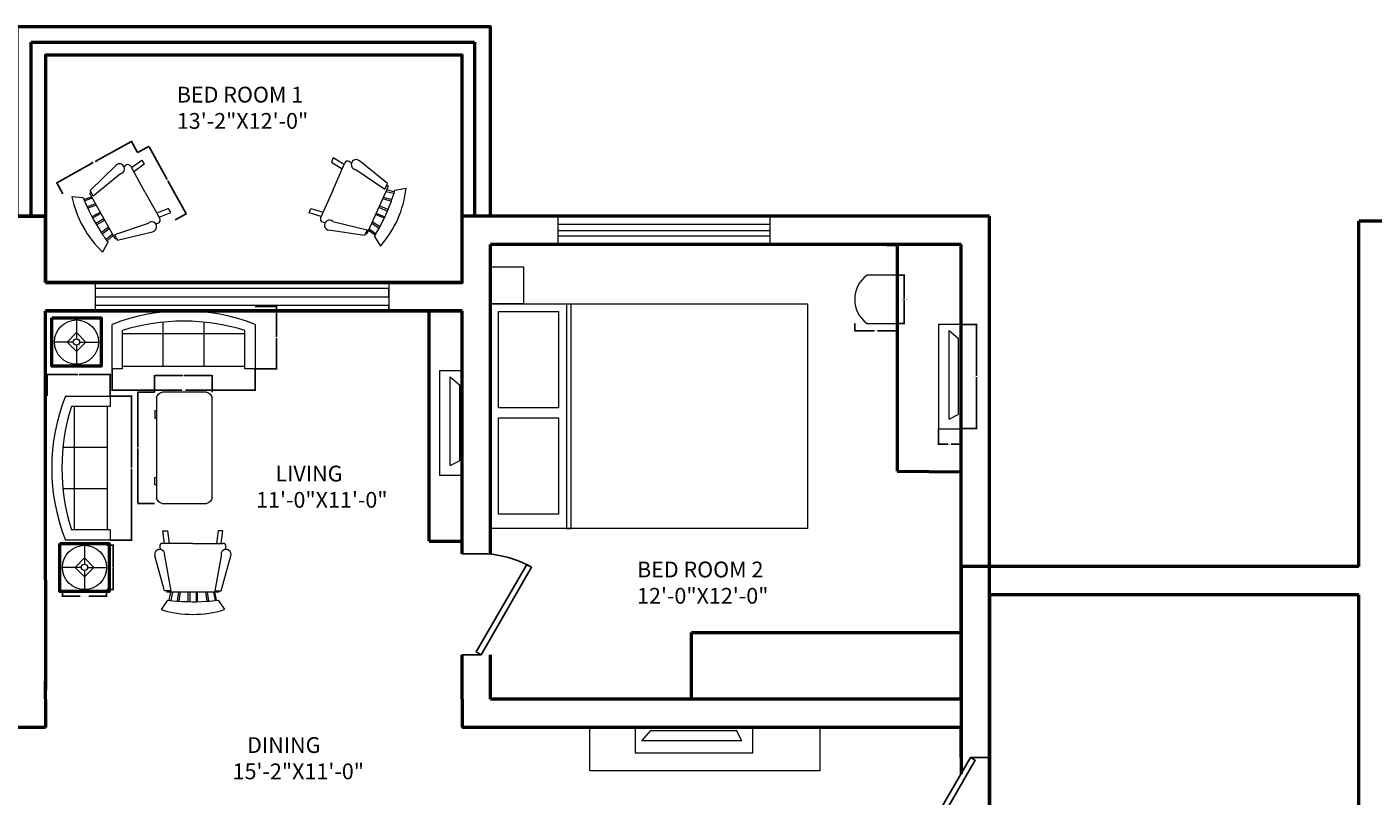
# Model space of a CAD drawing. Units: inches. Extents: x -105 to 1531, y -656 to 2003.
# Tile 5 of 6: x 553 to 979, y 856 to 1100. Entities that reach past the tile are written whole.
import ezdxf

# ---------------------------------------------------------------- set-up
doc = ezdxf.new("R2010")
doc.units = ezdxf.units.IN
doc.header["$MEASUREMENT"] = 0
for name, color, linetype, lineweight in [('A-ANNO-DIMS', 2, 'Continuous', 18), ('A-AREA-IDEN', 7, 'Continuous', 25), ('A-DOOR', 3, 'Continuous', 25), ('A-FURN', 8, 'Continuous', 18), ('A-GLAZ', 4, 'Continuous', 18), ('A-WALL', 7, 'Continuous', 50)]:
    doc.layers.add(name, color=color, linetype=linetype, lineweight=lineweight)
doc.styles.get("Standard").update_dxf_attribs({"font": 'arial.ttf'})
doc.dimstyles.get("Standard").update_dxf_attribs({"dimtxt": 0.18, "dimasz": 0.18, "dimexe": 0.18, "dimexo": 0.0625, "dimgap": 0.09, "dimtad": 0, "dimtih": 1, "dimtoh": 1, "dimdec": 0, "dimzin": 0, "dimdsep": 46, "dimlunit": 3, "dimtxsty": 'Standard', "dimcen": 0.09, "dimadec": 0, "dimazin": 0, "dimtfac": 1, "dimtdec": 0, "dimtofl": 0, "dimtmove": 0, "dimatfit": 3, "dimfxl": 1, "dimtolj": 1, "dimtzin": 0, "dimarcsym": 0})

# ---------------------------------------------------------------- blocks, each defined once
blk = doc.blocks.new('*U9')
for p, q in [((-32, 0), (-32, -6)), ((0, 0), (0, -6))]:
    blk.add_line(p, q)
blk.add_lwpolyline([(0, 0), (-27.71, 16), (-28.59, 14.48), (-0.88, -1.52)], close=True)
blk.add_arc((0, 0), 32, 150, 180)
blk = doc.blocks.new('Chair - Rocking')
for p, q in [((-8, -4.5), (-10, -1.5)), ((-4.5, -7), (-4.96674, -4.19951)), ((-4, -7), (-4.40532, -4.16272)), ((-1.5, -4.05012), (-1.5, -7)), ((-1, -7), (-1, -4.05012)), ((1, -7), (1, -4.04655)), ((1.5, -4.05012), (1.5, -7)), ((4, -7), (4.40187, -4.18694)), ((4.5, -7), (4.96761, -4.19437)), ((8, -4.5), (10, -1.5)), ((-9, -7.5), (-12, -18.49999)), ((-7, -7.5), (-9, -7.5)), ((-9, -18.49999), (-7, -7.5)), ((-8.23428, -6.99939), (-8.3093, -7.47958)), ((-8.23041, -7), (8.23915, -7)), ((-7.5, -4.5), (-7, -7)), ((-6.5, -7), (-7.02225, -4.43)), ((6.5, -7), (7, -4.4057)), ((7.5, -4.5), (7, -7)), ((7, -7.5), (9, -7.5)), ((9, -18.49999), (7, -7.5)), ((8.31071, -7.48854), (8.23449, -7.00073)), ((9, -7.5), (12, -18.49999)), ((-10.36644, -20.64523), (-10.5, -21.49999)), ((10.5, -21.49999), (10.3575, -20.58798)), ((-9, -22.49999), (-9.5, -26.49999)), ((0, -22.49999), (-9.5, -22.49999)), ((-8, -26.49999), (-7.5, -22.49999)), ((0, -22.49999), (9.5, -22.49999)), ((8, -26.49999), (7.5, -22.49999)), ((9, -22.49999), (9.5, -26.49999)), ((-9.5, -26.49999), (-8, -26.49999)), ((9.5, -26.49999), (8, -26.49999))]:
    blk.add_line(p, q)
for centre, radius, start, end in [((0, -34.08333), 34.08333, 72.93847, 107.0615), ((0, -68.25004), 64.25, 93.92211, 97.15267), ((0, -68.25004), 64.25, 82.84733, 93.92211), ((-10.5, -18.99999), 1.58114, 161.5651, 18.43495), ((10.5, -18.99999), 1.58114, 161.5651, 18.43495), ((-9.5, -21.49999), 1, 180, 270), ((9.5, -21.49999), 1, 270, 0)]:
    blk.add_arc(centre, radius, start, end)
blk = doc.blocks.new('Sofa - Roundback 7 ft.')
for p, q in [((-12.00002, -32.4421), (-12.00003, -6.5971)), ((11.99997, -32.4421), (11.99998, -6.5971)), ((-36.000027, -34), (-36.000027, -11.4696)), ((-35.999844, -13.3819), (35.9998, -13.3819)), ((35.99998, -34), (35.99998, -11.4696)), ((-36.000027, -32.4421), (35.99998, -32.4421))]:
    blk.add_line(p, q)
for points in [[(-36.000027, -34), (-42.000027, -34), (-42.000027, -8)], [(41.99998, -8), (41.99998, -34), (35.99998, -34)]]:
    blk.add_lwpolyline(points)
for centre, radius, start, end in [((0, -114.25), 114.25, 68.43141, 111.5686), ((-0.00001, -127.1968), 121.1968, 72.72033, 107.2797)]:
    blk.add_arc(centre, radius, start, end)
blk = doc.blocks.new('Desk - 30 x 60 in.')
for p, q in [((-26.999995, 0), (26.999995, 0)), ((-29.999995, -27), (-29.999995, -3)), ((29.999995, -3), (29.999995, -27)), ((26.999995, -30), (-26.999995, -30)), ((-20.000005, -30), (-20.000005, -31)), ((-20.000005, -31), (-16.000005, -31)), ((-16.000005, -31), (-16.000005, -30)), ((15.999995, -31), (15.999995, -30)), ((19.999995, -31), (15.999995, -31)), ((19.999995, -30), (19.999995, -31))]:
    blk.add_line(p, q)
for centre, start, end in [((-26.499995, -3.5), 98.1301, 171.8699), ((26.499995, -3.5), 8.130102, 81.8699), ((-26.499995, -26.5), 188.1301, 261.8699), ((26.499995, -26.5), 278.1301, 351.8699)]:
    blk.add_arc(centre, 3.535534, start, end)
blk = doc.blocks.new('Lamp - Table')
for p, q in [((0, 7), (0, 1)), ((-1, 0), (-7, 0)), ((0, 3), (-3, 0)), ((-3, 0), (0, -3)), ((3, 0), (0, 3)), ((0, -3), (3, 0)), ((1, 0), (7, 0)), ((0, -1), (0, -7))]:
    blk.add_line(p, q)
for radius in [7, 1]:
    blk.add_circle((0, 0), radius)
blk = doc.blocks.new('*U11')
for p, q in [((0, 0), (0, 6)), ((32, 0), (32, 6))]:
    blk.add_line(p, q)
blk.add_lwpolyline([(0, 0), (27.71, -16), (28.59, -14.48), (0.88, 1.52)], close=True)
blk.add_arc((0, 0), 32, 330, 0)
blk = doc.blocks.new('FURN-SIDE-TABLE')
for p, q in [((13.4, 15.25), (3.8, 15.25)), ((13.4, 0), (13.4, 15.25)), ((3.8, 0), (13.4, 0))]:
    blk.add_line(p, q)
blk.add_arc((9.55, 7.62), 9.55, 127.0288, 232.9712)
blk = doc.blocks.new('FURN-WALL-UNIT')
for p, q in [((3.37, 3.06), (3.37, 31.15)), ((3.37, 31.15), (6.26, 28.66)), ((6.26, 28.66), (6.26, 4.54)), ((3.37, 3.06), (6.26, 4.54))]:
    blk.add_line(p, q)
blk.add_lwpolyline([(7.13, 33.03), (0, 33.03), (0, 0), (7.13, 0)], close=True)
blk = doc.blocks.new('*D17')
at = {"layer": 'A-ANNO-DIMS', "color": 0, "lineweight": -2, "transparency": 16777216}
for p, q in [((586.1, 1063.19), (574.78, 1056.91)), ((588.19, 1059.79), (586.17, 1063.44)), ((562.8, 1050.27), (574.12, 1056.55)), ((564.58, 1046.7), (562.56, 1050.34))]:
    blk.add_line(p, q, dxfattribs=at)
at = {"layer": 'A-ANNO-DIMS', "color": 0, "transparency": 16777216}
for points in [[(586.08, 1063.22), (586.11, 1063.16), (586.26, 1063.28)], [(562.79, 1050.3), (562.82, 1050.25), (562.64, 1050.19)]]:
    blk.add_solid(points, dxfattribs=at)
at = {"layer": 'Defpoints', "color": 0, "transparency": 16777216}
for p in [(588.22, 1059.74), (562.64, 1050.19), (564.61, 1046.64)]:
    blk.add_point(p, dxfattribs=at)
at = {"layer": 'A-ANNO-DIMS', "color": 0, "transparency": 16777216, "insert": (574.45, 1056.73), "char_height": 0.18, "attachment_point": 5}
blk.add_mtext('\\A1;ROCKING CHAIR 27 TYP.', dxfattribs=at)
blk = doc.blocks.new('*D18')
at = {"layer": 'A-ANNO-DIMS', "color": 0, "lineweight": -2, "transparency": 16777216}
for p, q in [((588.28, 1059.77), (591.92, 1061.79)), ((591.85, 1061.54), (597.59, 1051.2)), ((603.52, 1040.49), (597.79, 1050.83)), ((600.12, 1038.4), (603.77, 1040.42))]:
    blk.add_line(p, q, dxfattribs=at)
at = {"layer": 'A-ANNO-DIMS', "color": 0, "transparency": 16777216}
for points in [[(591.88, 1061.56), (591.82, 1061.53), (591.76, 1061.7)], [(603.55, 1040.5), (603.5, 1040.47), (603.61, 1040.33)]]:
    blk.add_solid(points, dxfattribs=at)
at = {"layer": 'Defpoints', "color": 0, "transparency": 16777216}
for p in [(591.76, 1061.7), (588.22, 1059.74), (600.07, 1038.37)]:
    blk.add_point(p, dxfattribs=at)
at = {"layer": 'A-ANNO-DIMS', "color": 0, "transparency": 16777216, "insert": (597.69, 1051.01), "char_height": 0.18, "attachment_point": 5}
blk.add_mtext('\\A1;24 TYP.', dxfattribs=at)
blk = doc.blocks.new('*D19')
at = {"layer": 'A-ANNO-DIMS', "color": 0, "lineweight": -2, "transparency": 16777216}
for p, q in [((564.4, 921.22), (564.4, 919)), ((578.4, 921.22), (578.4, 919)), ((564.58, 919.18), (570.06, 919.18)), ((578.22, 919.18), (572.74, 919.18))]:
    blk.add_line(p, q, dxfattribs=at)
at = {"layer": 'A-ANNO-DIMS', "color": 0, "transparency": 16777216}
for points in [[(564.58, 919.21), (564.58, 919.15), (564.4, 919.18)], [(578.22, 919.21), (578.22, 919.15), (578.4, 919.18)]]:
    blk.add_solid(points, dxfattribs=at)
at = {"layer": 'Defpoints', "color": 0, "transparency": 16777216}
for p in [(564.4, 921.28), (578.4, 921.28), (578.4, 919.18)]:
    blk.add_point(p, dxfattribs=at)
at = {"layer": 'A-ANNO-DIMS', "color": 0, "transparency": 16777216, "insert": (571.4, 919.18), "char_height": 0.18, "attachment_point": 5}
blk.add_mtext('\\A1;TABLE LAMP 14 TYP.', dxfattribs=at)
blk = doc.blocks.new('*D20')
at = {"layer": 'A-ANNO-DIMS', "color": 0, "lineweight": -2, "transparency": 16777216}
for p, q in [((578.46, 935.28), (580.68, 935.28)), ((580.5, 935.1), (580.5, 928.46)), ((580.5, 921.46), (580.5, 928.1)), ((578.46, 921.28), (580.68, 921.28))]:
    blk.add_line(p, q, dxfattribs=at)
at = {"layer": 'A-ANNO-DIMS', "color": 0, "transparency": 16777216}
for points in [[(580.47, 935.1), (580.53, 935.1), (580.5, 935.28)], [(580.47, 921.46), (580.53, 921.46), (580.5, 921.28)]]:
    blk.add_solid(points, dxfattribs=at)
at = {"layer": 'Defpoints', "color": 0, "transparency": 16777216}
for p in [(578.4, 935.28), (580.5, 935.28), (578.4, 921.28)]:
    blk.add_point(p, dxfattribs=at)
at = {"layer": 'A-ANNO-DIMS', "color": 0, "transparency": 16777216, "insert": (580.5, 928.28), "char_height": 0.18, "attachment_point": 5}
blk.add_mtext('\\A1;14 TYP.', dxfattribs=at)
blk = doc.blocks.new('*D21')
at = {"layer": 'A-ANNO-DIMS', "color": 0, "lineweight": -2, "transparency": 16777216}
for p, q in [((579.55, 982.57), (586.51, 982.57)), ((586.33, 982.39), (586.33, 959.93)), ((586.33, 937.12), (586.33, 959.57)), ((579.55, 936.94), (586.51, 936.94))]:
    blk.add_line(p, q, dxfattribs=at)
at = {"layer": 'A-ANNO-DIMS', "color": 0, "transparency": 16777216}
for points in [[(586.3, 982.39), (586.36, 982.39), (586.33, 982.57)], [(586.3, 937.12), (586.36, 937.12), (586.33, 936.94)]]:
    blk.add_solid(points, dxfattribs=at)
at = {"layer": 'Defpoints', "color": 0, "transparency": 16777216}
for p in [(579.48, 982.57), (586.33, 982.57), (579.48, 936.94)]:
    blk.add_point(p, dxfattribs=at)
at = {"layer": 'A-ANNO-DIMS', "color": 0, "transparency": 16777216, "insert": (586.33, 959.75), "char_height": 0.18, "attachment_point": 5}
blk.add_mtext('\\A1;SOFA 46', dxfattribs=at)
blk = doc.blocks.new('*D22')
at = {"layer": 'A-ANNO-DIMS', "color": 0, "lineweight": -2, "transparency": 16777216}
for p, q in [((559.56, 982.63), (559.56, 989.59)), ((559.74, 989.41), (569.3, 989.41)), ((579.3, 989.41), (569.74, 989.41)), ((579.48, 982.63), (579.48, 989.59))]:
    blk.add_line(p, q, dxfattribs=at)
at = {"layer": 'A-ANNO-DIMS', "color": 0, "transparency": 16777216}
for points in [[(559.74, 989.44), (559.74, 989.38), (559.56, 989.41)], [(579.3, 989.44), (579.3, 989.38), (579.48, 989.41)]]:
    blk.add_solid(points, dxfattribs=at)
at = {"layer": 'Defpoints', "color": 0, "transparency": 16777216}
for p in [(559.56, 989.41), (559.56, 982.57), (579.48, 982.57)]:
    blk.add_point(p, dxfattribs=at)
at = {"layer": 'A-ANNO-DIMS', "color": 0, "transparency": 16777216, "insert": (569.52, 989.41), "char_height": 0.18, "attachment_point": 5}
blk.add_mtext('\\A1;20', dxfattribs=at)
blk = doc.blocks.new('*D23')
at = {"layer": 'A-ANNO-DIMS', "color": 0, "lineweight": -2, "transparency": 16777216}
for p, q in [((580.16, 991.18), (580.16, 984.27)), ((625.44, 991.18), (625.44, 984.27)), ((580.34, 984.45), (602.2, 984.45)), ((625.26, 984.45), (603.39, 984.45))]:
    blk.add_line(p, q, dxfattribs=at)
at = {"layer": 'A-ANNO-DIMS', "color": 0, "transparency": 16777216}
for points in [[(580.34, 984.48), (580.34, 984.42), (580.16, 984.45)], [(625.26, 984.48), (625.26, 984.42), (625.44, 984.45)]]:
    blk.add_solid(points, dxfattribs=at)
at = {"layer": 'Defpoints', "color": 0, "transparency": 16777216}
for p in [(580.16, 991.24), (625.44, 991.24), (625.44, 984.45)]:
    blk.add_point(p, dxfattribs=at)
at = {"layer": 'A-ANNO-DIMS', "color": 0, "transparency": 16777216, "insert": (602.8, 984.45), "char_height": 0.18, "attachment_point": 5}
blk.add_mtext('\\A1;SOFA 45', dxfattribs=at)
blk = doc.blocks.new('*D24')
at = {"layer": 'A-ANNO-DIMS', "color": 0, "lineweight": -2, "transparency": 16777216}
for p, q in [((625.5, 1011), (632.41, 1011)), ((632.23, 1010.82), (632.23, 1001.3)), ((632.23, 991.42), (632.23, 1000.94)), ((625.5, 991.24), (632.41, 991.24))]:
    blk.add_line(p, q, dxfattribs=at)
at = {"layer": 'A-ANNO-DIMS', "color": 0, "transparency": 16777216}
for points in [[(632.2, 1010.82), (632.26, 1010.82), (632.23, 1011)], [(632.2, 991.42), (632.26, 991.42), (632.23, 991.24)]]:
    blk.add_solid(points, dxfattribs=at)
at = {"layer": 'Defpoints', "color": 0, "transparency": 16777216}
for p in [(625.44, 1011), (632.23, 1011), (625.44, 991.24)]:
    blk.add_point(p, dxfattribs=at)
at = {"layer": 'A-ANNO-DIMS', "color": 0, "transparency": 16777216, "insert": (632.23, 1001.12), "char_height": 0.18, "attachment_point": 5}
blk.add_mtext('\\A1;20', dxfattribs=at)
blk = doc.blocks.new('*D31')
at = {"layer": 'A-ANNO-DIMS', "color": 0, "lineweight": -2, "transparency": 16777216}
for p, q in [((828.81, 1020.84), (831.21, 1020.84)), ((831.03, 1020.66), (831.03, 1013.4)), ((831.03, 1005.77), (831.03, 1013.03)), ((828.81, 1005.59), (831.21, 1005.59))]:
    blk.add_line(p, q, dxfattribs=at)
at = {"layer": 'A-ANNO-DIMS', "color": 0, "transparency": 16777216}
for points in [[(831, 1020.66), (831.06, 1020.66), (831.03, 1020.84)], [(831, 1005.77), (831.06, 1005.77), (831.03, 1005.59)]]:
    blk.add_solid(points, dxfattribs=at)
at = {"layer": 'Defpoints', "color": 0, "transparency": 16777216}
for p in [(828.74, 1020.84), (831.03, 1020.84), (828.74, 1005.59)]:
    blk.add_point(p, dxfattribs=at)
at = {"layer": 'A-ANNO-DIMS', "color": 0, "transparency": 16777216, "insert": (831.03, 1013.21), "char_height": 0.18, "attachment_point": 5}
blk.add_mtext('\\A1;SIDE TABLE 15 TYP.', dxfattribs=at)
blk = doc.blocks.new('*D32')
at = {"layer": 'A-ANNO-DIMS', "color": 0, "lineweight": -2, "transparency": 16777216}
for p, q in [((815.34, 1005.53), (815.34, 1003.12)), ((815.52, 1003.3), (821.52, 1003.3)), ((828.56, 1003.3), (822.56, 1003.3)), ((828.74, 1005.53), (828.74, 1003.12))]:
    blk.add_line(p, q, dxfattribs=at)
at = {"layer": 'A-ANNO-DIMS', "color": 0, "transparency": 16777216}
for points in [[(815.52, 1003.33), (815.52, 1003.27), (815.34, 1003.3)], [(828.56, 1003.33), (828.56, 1003.27), (828.74, 1003.3)]]:
    blk.add_solid(points, dxfattribs=at)
at = {"layer": 'Defpoints', "color": 0, "transparency": 16777216}
for p in [(815.34, 1005.59), (828.74, 1005.59), (828.74, 1003.3)]:
    blk.add_point(p, dxfattribs=at)
at = {"layer": 'A-ANNO-DIMS', "color": 0, "transparency": 16777216, "insert": (822.04, 1003.3), "char_height": 0.18, "attachment_point": 5}
blk.add_mtext('\\A1;13 TYP.', dxfattribs=at)
blk = doc.blocks.new('*D33')
at = {"layer": 'A-ANNO-DIMS', "color": 0, "lineweight": -2, "transparency": 16777216}
for p, q in [((593.56, 983.78), (588.16, 983.78)), ((588.34, 983.6), (588.34, 966.35)), ((588.34, 948.74), (588.34, 965.98)), ((593.56, 948.56), (588.16, 948.56))]:
    blk.add_line(p, q, dxfattribs=at)
at = {"layer": 'A-ANNO-DIMS', "color": 0, "transparency": 16777216}
for points in [[(588.31, 983.6), (588.37, 983.6), (588.34, 983.78)], [(588.31, 948.74), (588.37, 948.74), (588.34, 948.56)]]:
    blk.add_solid(points, dxfattribs=at)
at = {"layer": 'Defpoints', "color": 0, "transparency": 16777216}
for p in [(588.34, 983.78), (593.62, 983.78), (593.62, 948.56)]:
    blk.add_point(p, dxfattribs=at)
at = {"layer": 'A-ANNO-DIMS', "color": 0, "transparency": 16777216, "insert": (588.34, 966.17), "char_height": 0.18, "attachment_point": 5}
blk.add_mtext('\\A1;TABLE 35', dxfattribs=at)
blk = doc.blocks.new('*D34')
at = {"layer": 'A-ANNO-DIMS', "color": 0, "lineweight": -2, "transparency": 16777216}
for p, q in [((593.62, 983.84), (593.62, 989.24)), ((611.82, 983.84), (611.82, 989.24)), ((593.8, 989.06), (602.51, 989.06)), ((611.64, 989.06), (602.93, 989.06))]:
    blk.add_line(p, q, dxfattribs=at)
at = {"layer": 'A-ANNO-DIMS', "color": 0, "transparency": 16777216}
for points in [[(593.8, 989.09), (593.8, 989.03), (593.62, 989.06)], [(611.64, 989.09), (611.64, 989.03), (611.82, 989.06)]]:
    blk.add_solid(points, dxfattribs=at)
at = {"layer": 'Defpoints', "color": 0, "transparency": 16777216}
for p in [(611.82, 989.06), (593.62, 983.78), (611.82, 983.78)]:
    blk.add_point(p, dxfattribs=at)
at = {"layer": 'A-ANNO-DIMS', "color": 0, "transparency": 16777216, "insert": (602.72, 989.06), "char_height": 0.18, "attachment_point": 5}
blk.add_mtext('\\A1;18', dxfattribs=at)
blk = doc.blocks.new('*D37')
at = {"layer": 'A-ANNO-DIMS', "color": 0, "lineweight": -2, "transparency": 16777216}
for p, q in [((849.06, 1005.28), (854.13, 1005.28)), ((853.95, 1005.1), (853.95, 988.94)), ((853.95, 972.43), (853.95, 988.58)), ((849.06, 972.25), (854.13, 972.25))]:
    blk.add_line(p, q, dxfattribs=at)
at = {"layer": 'A-ANNO-DIMS', "color": 0, "transparency": 16777216}
for points in [[(853.92, 1005.1), (853.98, 1005.1), (853.95, 1005.28)], [(853.92, 972.43), (853.98, 972.43), (853.95, 972.25)]]:
    blk.add_solid(points, dxfattribs=at)
at = {"layer": 'Defpoints', "color": 0, "transparency": 16777216}
for p in [(849, 1005.28), (853.95, 1005.28), (849, 972.25)]:
    blk.add_point(p, dxfattribs=at)
at = {"layer": 'A-ANNO-DIMS', "color": 0, "transparency": 16777216, "insert": (853.95, 988.76), "char_height": 0.18, "attachment_point": 5}
blk.add_mtext('\\A1;WALL UNIT 33 TYP.', dxfattribs=at)
blk = doc.blocks.new('*D38')
at = {"layer": 'A-ANNO-DIMS', "color": 0, "lineweight": -2, "transparency": 16777216}
for p, q in [((841.87, 972.18), (841.87, 967.11)), ((849, 972.18), (849, 967.11)), ((842.05, 967.29), (844.98, 967.29)), ((848.82, 967.29), (845.89, 967.29))]:
    blk.add_line(p, q, dxfattribs=at)
at = {"layer": 'A-ANNO-DIMS', "color": 0, "transparency": 16777216}
for points in [[(842.05, 967.32), (842.05, 967.26), (841.87, 967.29)], [(848.82, 967.32), (848.82, 967.26), (849, 967.29)]]:
    blk.add_solid(points, dxfattribs=at)
at = {"layer": 'Defpoints', "color": 0, "transparency": 16777216}
for p in [(841.87, 972.25), (849, 972.25), (849, 967.29)]:
    blk.add_point(p, dxfattribs=at)
at = {"layer": 'A-ANNO-DIMS', "color": 0, "transparency": 16777216, "insert": (845.44, 967.29), "char_height": 0.18, "attachment_point": 5}
blk.add_mtext('\\A1;7 TYP.', dxfattribs=at)

msp = doc.modelspace()

# ---------------------------------------------------------------- linework, layer by layer
at = {"layer": 'A-FURN'}
for p, q in [((724.04, 1011.81), (724.04, 940.63)), ((725.55, 940.63), (725.55, 1011.81)), ((724.04, 940.63), (725.55, 940.63)), ((747.92, 873.33), (750.73, 876.59)), ((750.73, 876.59), (777.92, 876.59)), ((779.59, 873.33), (777.92, 876.59)), ((779.59, 873.33), (747.92, 873.33))]:
    msp.add_line(p, q, dxfattribs=at)
for points in [[(700, 1023.5), (710.46, 1023.5), (710.46, 1011.81), (700, 1011.81)], [(700, 1011.81), (800.4, 1011.81), (800.4, 940.63), (700, 940.63)], [(702.55, 1009.35), (721.55, 1009.35), (721.55, 978.86), (702.55, 978.86)], [(702.55, 975.68), (721.55, 975.68), (721.55, 945.2), (702.55, 945.2)], [(731.49, 877.57), (804.33, 877.57), (804.33, 863.82), (731.49, 863.82)], [(745.8, 877.57), (745.8, 869.53), (783.04, 869.53), (783.04, 877.57)]]:
    msp.add_lwpolyline(points, close=True, dxfattribs=at)
at = {"layer": 'A-GLAZ'}
for p, q in [((721.39, 1030.57), (721.39, 1039.57)), ((721.39, 1039.57), (788.5, 1039.57)), ((721.39, 1037.08), (788.5, 1037.08)), ((788.5, 1039.57), (788.5, 1030.57)), ((788.5, 1037.08), (788.5, 1033.3)), ((721.39, 1033.3), (721.39, 1035.07)), ((721.39, 1035.07), (788.5, 1035.07)), ((788.5, 1033.3), (721.39, 1033.3)), ((788.5, 1030.57), (721.39, 1030.57)), ((574.9, 1009.57), (574.9, 1018.57)), ((574.9, 1018.57), (667.83, 1018.57)), ((667.83, 1016.65), (574.9, 1016.65)), ((667.83, 1018.57), (667.83, 1009.57)), ((667.83, 1014.07), (667.83, 1016.65)), ((574.9, 1011.29), (574.9, 1014.07)), ((574.9, 1014.07), (667.83, 1014.07)), ((667.83, 1011.29), (574.9, 1011.29)), ((667.83, 1009.57), (667.83, 1011.29))]:
    msp.add_line(p, q, dxfattribs=at)
at = {"layer": 'A-WALL'}
for p, q in [((554.5, 1039.57), (554.5, 1094.72)), ((554.5, 1094.72), (694.89, 1094.72)), ((694.89, 1094.72), (694.89, 1039.57)), ((691, 1018.57), (691, 1090.57)), ((559, 1039.57), (383, 1039.57)), ((550, 1039.57), (559, 1039.57)), ((559, 1039.57), (554.5, 1039.57)), ((559, 1018.57), (559, 1039.57)), ((858, 1039.57), (691, 1039.57)), ((691, 1018.57), (691, 1039.57)), ((858, 743.57), (858, 1039.57)), ((1128, 1037.97), (975, 1037.97)), ((975, 928.57), (975, 1037.97)), ((849, 1030.57), (700, 1030.57)), ((700, 932.46), (700, 1030.57)), ((825.45, 1030.57), (828.74, 1030.57)), ((828.74, 1030.57), (828.74, 958.78)), ((849, 886.57), (849, 1030.57)), ((691, 1018.57), (559, 1018.57)), ((691, 1009.57), (559, 1009.57)), ((559, 924.27), (559, 1009.57)), ((680.54, 936.55), (680.54, 1009.57)), ((691, 932.6), (691, 1009.57)), ((828.74, 958.78), (849, 958.57)), ((680.54, 936.55), (691, 936.55)), ((559, 924.27), (559, 889.42)), ((975, 743.57), (975, 919.57)), ((975, 625.97), (975, 919.57)), ((763.61, 886.57), (763.61, 907.68)), ((763.61, 907.68), (849, 907.68)), ((691, 886.57), (691, 900.6)), ((700, 886.57), (700, 900.6)), ((559, 886.57), (559, 892.27)), ((559, 886.57), (559, 877.57)), ((691, 886.57), (691, 877.57)), ((849, 886.57), (700, 886.57)), ((559, 877.57), (547.42, 877.57)), ((849, 877.57), (691, 877.57)), ((849, 868.07), (849, 877.57)), ((849, 868.07), (849, 862.87))]:
    msp.add_line(p, q, dxfattribs=at)
for points in [[(700, 1039.57), (700, 1099.57), (550, 1099.57), (550, 1039.57)], [(700, 1009.57), (700, 1030.57)], [(559, 1009.57), (691, 1009.57)], [(975, 928.57), (849, 928.57), (849, 868.07)], [(975, 919.57), (858, 919.57), (858, 743.57), (975, 743.57)]]:
    msp.add_lwpolyline(points, dxfattribs=at)
for points in [[(559, 1018.57), (691, 1018.57), (691, 1090.57), (559, 1090.57)], [(561.08, 1007.33), (576.65, 1007.33), (576.65, 992.07), (561.08, 992.07)], [(563.61, 935.91), (579.18, 935.91), (579.18, 920.65), (563.61, 920.65)]]:
    msp.add_lwpolyline(points, close=True, dxfattribs=at)

# ---------------------------------------------------------------- block references
at = {"layer": 'A-DOOR', "rotation": 270}
for name, p in [('*U9', (697, 900.6)), ('*U11', (852, 868.07))]:
    msp.add_blockref(name, p, dxfattribs=at)
at = {"layer": 'A-FURN'}
for p, rotation in [((570.97, 1036.2), 119.0073306236213), ((670.6, 1038.66), 246.1612300702624), ((605.72, 913.4), 179.9999822143792)]:
    msp.add_blockref('Chair - Rocking', p, dxfattribs=dict(at, rotation=rotation))
for name, p in [('FURN-SIDE-TABLE', (815.34, 1005.59)), ('Lamp - Table', (568.86, 999.7)), ('FURN-WALL-UNIT', (841.87, 972.24)), ('FURN-WALL-UNIT', (683.87, 957.51)), ('Lamp - Table', (571.4, 928.28))]:
    msp.add_blockref(name, p, dxfattribs=at)
at = {"layer": 'A-FURN', "xscale": 0.5390846654517311, "yscale": 0.5390846654517311, "zscale": 0.5390846654517311}
msp.add_blockref('Sofa - Roundback 7 ft.', (602.8, 1009.57), dxfattribs=at)
at = {"layer": 'A-FURN'}
for name, p, xscale, yscale, zscale, rotation in [('Sofa - Roundback 7 ft.', (561.01, 959.75), 0.5432271373160069, 0.5432271373160069, 0.5432271373160069, 90), ('Desk - 30 x 60 in.', (611.82, 966.17), -0.586967752190793, 0.586967752190793, 0.586967752190793, 270)]:
    msp.add_blockref(name, p, dxfattribs=dict(at, xscale=xscale, yscale=yscale, zscale=zscale, rotation=rotation))

# ---------------------------------------------------------------- texts
at = {"layer": 'A-AREA-IDEN', "ltscale": 5, "char_height": 5, "attachment_point": 1}
for s, insert in [('BED ROOM 1\\P13\'-2"X12\'-0"', (600.63, 1080.61)), ('    LIVING\\P11\'-0"X11\'-0"', (625.75, 960.52)), ('BED ROOM 2\\P12\'-0"X12\'-0"', (746.39, 930.12)), ('   DINING\\P15\'-2"X11\'-0"', (618.3, 874.48))]:
    msp.add_mtext_dynamic_manual_height_columns(s, width=114.6643, gutter_width=1, heights=[0], dxfattribs=dict(at, insert=insert))

# ---------------------------------------------------------------- dimensions: what is measured, and where the dimension line sits
at = {"layer": 'A-ANNO-DIMS'}
for base, p1, p2, angle, text, picture, middle in [((562.64, 1050.19), (588.22, 1059.74), (564.61, 1046.64), 209.0073, 'ROCKING CHAIR <> TYP.', '*D17', (574.45, 1056.73)), ((591.76, 1061.7), (600.07, 1038.37), (588.22, 1059.74), 119.0073, '<> TYP.', '*D18', (597.69, 1051.01)), ((831.03, 1020.84), (828.74, 1005.59), (828.74, 1020.84), 90, 'SIDE TABLE <> TYP.', '*D31', (831.03, 1013.21)), ((853.95, 1005.28), (849, 972.25), (849, 1005.28), 90, 'WALL UNIT <> TYP.', '*D37', (853.95, 988.76)), ((586.33, 982.57), (579.48, 936.94), (579.48, 982.57), 90, 'SOFA <>', '*D21', (586.33, 959.75)), ((588.34, 983.78), (593.62, 948.56), (593.62, 983.78), 90, 'TABLE <>', '*D33', (588.34, 966.17)), ((580.5, 935.28), (578.4, 921.28), (578.4, 935.28), 90, '<> TYP.', '*D20', (580.5, 928.28))]:
    dim = msp.add_linear_dim(base=base, p1=p1, p2=p2, angle=angle, text=text, dimstyle='Standard', override={"dimdec": 0, "dimlfac": 1, "dimrnd": 0, "dimzin": 0, "dimdsep": 46, "dimlunit": 2}, dxfattribs=at)
    dim.commit()
    dim.dimension.update_dxf_attribs({"geometry": picture, "text_midpoint": middle})
for base, p1, p2, angle, picture, middle in [((632.23, 1011), (625.44, 991.24), (625.44, 1011), 90, '*D24', (632.23, 1001.12)), ((559.56, 989.41), (579.48, 982.57), (559.56, 982.57), 180, '*D22', (569.52, 989.41))]:
    dim = msp.add_linear_dim(base=base, p1=p1, p2=p2, angle=angle, dimstyle='Standard', override={"dimdec": 0, "dimlfac": 1, "dimrnd": 0, "dimzin": 0, "dimdsep": 46, "dimlunit": 2}, dxfattribs=at)
    dim.commit()
    dim.dimension.update_dxf_attribs({"geometry": picture, "text_midpoint": middle})
for base, p1, p2, text, picture, middle in [((828.74, 1003.3), (815.34, 1005.59), (828.74, 1005.59), '<> TYP.', '*D32', (822.04, 1003.3)), ((625.44, 984.45), (580.16, 991.24), (625.44, 991.24), 'SOFA <>', '*D23', (602.8, 984.45)), ((849, 967.29), (841.87, 972.25), (849, 972.25), '<> TYP.', '*D38', (845.44, 967.29)), ((578.4, 919.18), (564.4, 921.28), (578.4, 921.28), 'TABLE LAMP <> TYP.', '*D19', (571.4, 919.18))]:
    dim = msp.add_linear_dim(base=base, p1=p1, p2=p2, text=text, dimstyle='Standard', override={"dimdec": 0, "dimlfac": 1, "dimrnd": 0, "dimzin": 0, "dimdsep": 46, "dimlunit": 2}, dxfattribs=at)
    dim.commit()
    dim.dimension.update_dxf_attribs({"geometry": picture, "text_midpoint": middle})
dim = msp.add_linear_dim(base=(611.82, 989.06), p1=(593.62, 983.78), p2=(611.82, 983.78), dimstyle='Standard', override={"dimdec": 0, "dimlfac": 1, "dimrnd": 0, "dimzin": 0, "dimdsep": 46, "dimlunit": 2}, dxfattribs=at)
dim.commit()
dim.dimension.update_dxf_attribs({"geometry": '*D34', "text_midpoint": (602.72, 989.06)})

doc.saveas('drawing.dxf')
